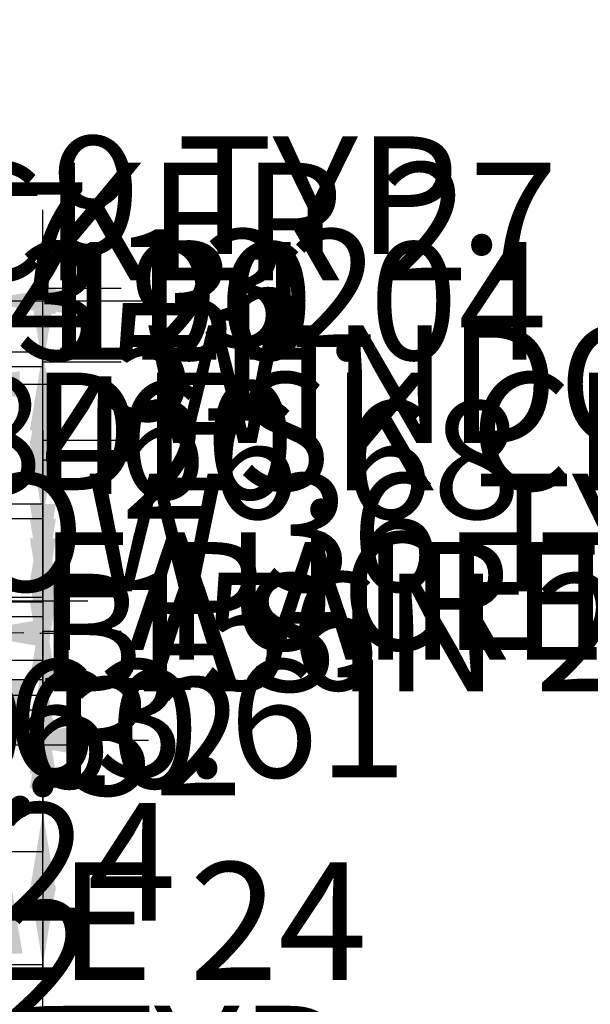
# Model space of a CAD drawing. Units: inches. Extents: x -307 to 2141, y -58 to 895.
# Tile 27 of 28: x 933 to 1283, y 292 to 895. Entities that reach past the tile are written whole.
import ezdxf

# ---------------------------------------------------------------- set-up
doc = ezdxf.new("R2010")
doc.units = ezdxf.units.IN
doc.header["$MEASUREMENT"] = 0
doc.layers.add('A-ANNO-DIMS', color=2, linetype='Continuous', lineweight=18)
doc.styles.get("Standard").update_dxf_attribs({"font": 'arial.ttf'})
doc.dimstyles.get("Standard").update_dxf_attribs({"dimtxt": 72, "dimasz": 48, "dimexe": 0.18, "dimexo": 0.0625, "dimgap": 0.09, "dimtad": 0, "dimtih": 1, "dimtoh": 1, "dimdec": 0, "dimrnd": 48, "dimzin": 0, "dimdsep": 46, "dimlunit": 3, "dimtxsty": 'Standard', "dimcen": 0.09, "dimadec": 0, "dimazin": 0, "dimtfac": 1, "dimtdec": 0, "dimtofl": 0, "dimtmove": 0, "dimatfit": 3, "dimfxl": 1, "dimtolj": 1, "dimtzin": 0, "dimarcsym": 0})

# ---------------------------------------------------------------- blocks, each defined once
blk = doc.blocks.new('*D29')
at = {"layer": 'A-ANNO-DIMS', "color": 0, "lineweight": -2, "transparency": 16777216}
for p, q in [((747.42, 450.87), (699.42, 450.87)), ((795.42, 433.61), (795.42, 451.05)), ((882.03, 433.61), (882.03, 451.05)), ((930.03, 450.87), (978.03, 450.87))]:
    blk.add_line(p, q, dxfattribs=at)
at = {"layer": 'A-ANNO-DIMS', "color": 0, "transparency": 16777216}
for points in [[(747.42, 458.87), (747.42, 442.87), (795.42, 450.87)], [(930.03, 458.87), (930.03, 442.87), (882.03, 450.87)]]:
    blk.add_solid(points, dxfattribs=at)
at = {"layer": 'Defpoints', "color": 0, "transparency": 16777216}
for p in [(795.42, 450.87), (795.42, 433.55), (882.03, 433.55)]:
    blk.add_point(p, dxfattribs=at)
at = {"layer": 'A-ANNO-DIMS', "color": 0, "transparency": 16777216, "insert": (647.71, 450.87), "char_height": 72, "attachment_point": 5}
blk.add_mtext('\\A1;87', dxfattribs=at)
blk = doc.blocks.new('*D30')
at = {"layer": 'A-ANNO-DIMS', "color": 0, "lineweight": -2, "transparency": 16777216}
for p, q in [((570.74, 532.83), (570.74, 580.83)), ((570.74, 580.83), (618.74, 580.83)), ((565.4, 484.83), (570.92, 484.83)), ((565.4, 448.83), (570.92, 448.83)), ((570.74, 400.83), (570.74, 352.83))]:
    blk.add_line(p, q, dxfattribs=at)
at = {"layer": 'A-ANNO-DIMS', "color": 0, "transparency": 16777216}
for points in [[(562.74, 532.83), (578.74, 532.83), (570.74, 484.83)], [(562.74, 400.83), (578.74, 400.83), (570.74, 448.83)]]:
    blk.add_solid(points, dxfattribs=at)
at = {"layer": 'Defpoints', "color": 0, "transparency": 16777216}
for p in [(565.34, 484.83), (570.74, 484.83), (565.34, 448.83)]:
    blk.add_point(p, dxfattribs=at)
at = {"layer": 'A-ANNO-DIMS', "color": 0, "transparency": 16777216, "insert": (1030.17, 580.83), "char_height": 72, "attachment_point": 5}
blk.add_mtext('\\A1;WINDOW 36 TYP.', dxfattribs=at)
blk = doc.blocks.new('*D31')
at = {"layer": 'A-ANNO-DIMS', "color": 0, "lineweight": -2, "transparency": 16777216}
for p, q in [((556.34, 448.77), (556.34, 443.25)), ((565.34, 448.77), (565.34, 443.25)), ((508.34, 443.43), (460.34, 443.43)), ((613.34, 443.43), (661.34, 443.43))]:
    blk.add_line(p, q, dxfattribs=at)
at = {"layer": 'A-ANNO-DIMS', "color": 0, "transparency": 16777216}
for points in [[(508.34, 451.43), (508.34, 435.43), (556.34, 443.43)], [(613.34, 451.43), (613.34, 435.43), (565.34, 443.43)]]:
    blk.add_solid(points, dxfattribs=at)
at = {"layer": 'Defpoints', "color": 0, "transparency": 16777216}
for p in [(556.34, 448.83), (565.34, 448.83), (565.34, 443.43)]:
    blk.add_point(p, dxfattribs=at)
at = {"layer": 'A-ANNO-DIMS', "color": 0, "transparency": 16777216, "insert": (808.69, 443.43), "char_height": 72, "attachment_point": 5}
blk.add_mtext('\\A1;9 TYP.', dxfattribs=at)
blk = doc.blocks.new('*D32')
at = {"layer": 'A-ANNO-DIMS', "color": 0, "lineweight": -2, "transparency": 16777216}
for p, q in [((813.29, 682.28), (813.29, 671.36)), ((885.29, 682.28), (885.29, 671.36)), ((765.29, 671.54), (717.29, 671.54)), ((933.29, 671.54), (981.29, 671.54))]:
    blk.add_line(p, q, dxfattribs=at)
at = {"layer": 'A-ANNO-DIMS', "color": 0, "transparency": 16777216}
for points in [[(765.29, 679.54), (765.29, 663.54), (813.29, 671.54)], [(933.29, 679.54), (933.29, 663.54), (885.29, 671.54)]]:
    blk.add_solid(points, dxfattribs=at)
at = {"layer": 'Defpoints', "color": 0, "transparency": 16777216}
for p in [(813.29, 682.34), (885.29, 682.34), (885.29, 671.54)]:
    blk.add_point(p, dxfattribs=at)
at = {"layer": 'A-ANNO-DIMS', "color": 0, "transparency": 16777216, "insert": (1392.73, 671.54), "char_height": 72, "attachment_point": 5}
blk.add_mtext('\\A1;WINDOW 72 TYP.', dxfattribs=at)
blk = doc.blocks.new('*D33')
at = {"layer": 'A-ANNO-DIMS', "color": 0, "lineweight": -2, "transparency": 16777216}
for p, q in [((896.09, 739.34), (896.09, 787.34)), ((896.09, 787.34), (944.09, 787.34)), ((885.36, 691.34), (896.27, 691.34)), ((885.36, 682.34), (896.27, 682.34)), ((896.09, 634.34), (896.09, 586.34))]:
    blk.add_line(p, q, dxfattribs=at)
at = {"layer": 'A-ANNO-DIMS', "color": 0, "transparency": 16777216}
for points in [[(888.09, 739.34), (904.09, 739.34), (896.09, 691.34)], [(888.09, 634.34), (904.09, 634.34), (896.09, 682.34)]]:
    blk.add_solid(points, dxfattribs=at)
at = {"layer": 'Defpoints', "color": 0, "transparency": 16777216}
for p in [(885.29, 691.34), (896.09, 691.34), (885.29, 682.34)]:
    blk.add_point(p, dxfattribs=at)
at = {"layer": 'A-ANNO-DIMS', "color": 0, "transparency": 16777216, "insert": (1091.45, 787.34), "char_height": 72, "attachment_point": 5}
blk.add_mtext('\\A1;9 TYP.', dxfattribs=at)
blk = doc.blocks.new('*D34')
at = {"layer": 'A-ANNO-DIMS', "color": 0, "lineweight": -2, "transparency": 16777216}
for p, q in [((927.14, 490.97), (927.14, 538.97)), ((927.14, 538.97), (975.14, 538.97)), ((916.4, 442.97), (927.32, 442.97)), ((916.4, 370.95), (927.32, 370.95)), ((927.14, 322.95), (927.14, 274.95))]:
    blk.add_line(p, q, dxfattribs=at)
at = {"layer": 'A-ANNO-DIMS', "color": 0, "transparency": 16777216}
for points in [[(919.14, 490.97), (935.14, 490.97), (927.14, 442.97)], [(919.14, 322.95), (935.14, 322.95), (927.14, 370.95)]]:
    blk.add_solid(points, dxfattribs=at)
at = {"layer": 'Defpoints', "color": 0, "transparency": 16777216}
for p in [(916.34, 442.97), (927.14, 442.97), (916.34, 370.95)]:
    blk.add_point(p, dxfattribs=at)
at = {"layer": 'A-ANNO-DIMS', "color": 0, "transparency": 16777216, "insert": (1584.53, 538.97), "char_height": 72, "attachment_point": 5}
blk.add_mtext('\\A1;PAIRED WINDOW 72 TYP.', dxfattribs=at)
blk = doc.blocks.new('*D35')
at = {"layer": 'A-ANNO-DIMS', "color": 0, "lineweight": -2, "transparency": 16777216}
for p, q in [((859.34, 453.77), (811.34, 453.77)), ((907.34, 443.03), (907.34, 453.95)), ((916.34, 443.03), (916.34, 453.95)), ((964.34, 453.77), (1012.34, 453.77))]:
    blk.add_line(p, q, dxfattribs=at)
at = {"layer": 'A-ANNO-DIMS', "color": 0, "transparency": 16777216}
for points in [[(859.34, 461.77), (859.34, 445.77), (907.34, 453.77)], [(964.34, 461.77), (964.34, 445.77), (916.34, 453.77)]]:
    blk.add_solid(points, dxfattribs=at)
at = {"layer": 'Defpoints', "color": 0, "transparency": 16777216}
for p in [(907.34, 453.77), (907.34, 442.97), (916.34, 442.97)]:
    blk.add_point(p, dxfattribs=at)
at = {"layer": 'A-ANNO-DIMS', "color": 0, "transparency": 16777216, "insert": (663.98, 453.77), "char_height": 72, "attachment_point": 5}
blk.add_mtext('\\A1;9 TYP.', dxfattribs=at)
blk = doc.blocks.new('*D37')
at = {"layer": 'A-ANNO-DIMS', "color": 0, "lineweight": -2, "transparency": 16777216}
for p, q in [((828.62, 519.41), (780.62, 519.46)), ((876.61, 514.46), (876.62, 519.54)), ((897.61, 514.44), (897.62, 519.51)), ((945.62, 519.28), (993.62, 519.22))]:
    blk.add_line(p, q, dxfattribs=at)
at = {"layer": 'A-ANNO-DIMS', "color": 0, "transparency": 16777216}
for points in [[(828.63, 527.41), (828.61, 511.41), (876.62, 519.36)], [(945.63, 527.28), (945.61, 511.28), (897.62, 519.33)]]:
    blk.add_solid(points, dxfattribs=at)
at = {"layer": 'Defpoints', "color": 0, "transparency": 16777216}
for p in [(876.62, 519.36), (876.61, 514.4), (897.61, 514.38)]:
    blk.add_point(p, dxfattribs=at)
at = {"layer": 'A-ANNO-DIMS', "color": 0, "transparency": 16777216, "insert": (604.68, 519.46), "char_height": 72, "attachment_point": 5}
blk.add_mtext('\\A1;21 TYP.', dxfattribs=at)
blk = doc.blocks.new('*D41')
at = {"layer": 'A-ANNO-DIMS', "color": 0, "lineweight": -2, "transparency": 16777216}
for p, q in [((768.38, 207.13), (768.38, 255.13)), ((768.38, 255.13), (816.38, 255.13)), ((762.83, 159.13), (768.56, 159.13)), ((762.83, 128.96), (768.56, 128.96)), ((768.38, 80.96), (768.38, 32.96))]:
    blk.add_line(p, q, dxfattribs=at)
at = {"layer": 'A-ANNO-DIMS', "color": 0, "transparency": 16777216}
for points in [[(760.38, 207.13), (776.38, 207.13), (768.38, 159.13)], [(760.38, 80.96), (776.38, 80.96), (768.38, 128.96)]]:
    blk.add_solid(points, dxfattribs=at)
at = {"layer": 'Defpoints', "color": 0, "transparency": 16777216}
for p in [(762.77, 159.13), (768.38, 159.13), (762.77, 128.96)]:
    blk.add_point(p, dxfattribs=at)
at = {"layer": 'A-ANNO-DIMS', "color": 0, "transparency": 16777216, "insert": (991.68, 255.13), "char_height": 72, "attachment_point": 5}
blk.add_mtext('\\A1;30 TYP.', dxfattribs=at)
blk = doc.blocks.new('*D42')
at = {"layer": 'A-ANNO-DIMS', "color": 0, "lineweight": -2, "transparency": 16777216}
for p, q in [((822.3, 541.2), (822.27, 542.82)), ((832.3, 541.41), (832.27, 543.03)), ((880.26, 543.86), (928.25, 544.87)), ((774.28, 541.63), (726.29, 540.62))]:
    blk.add_line(p, q, dxfattribs=at)
at = {"layer": 'A-ANNO-DIMS', "color": 0, "transparency": 16777216}
for points in [[(774.11, 549.63), (774.45, 533.63), (822.27, 542.64)], [(880.09, 551.86), (880.43, 535.86), (832.27, 542.85)]]:
    blk.add_solid(points, dxfattribs=at)
at = {"layer": 'Defpoints', "color": 0, "transparency": 16777216}
for p in [(832.27, 542.85), (822.3, 541.14), (832.3, 541.35)]:
    blk.add_point(p, dxfattribs=at)
at = {"layer": 'A-ANNO-DIMS', "color": 0, "transparency": 16777216, "insert": (1192.89, 544.87), "char_height": 72, "attachment_point": 5}
blk.add_mtext('\\A1;FAUCET 10', dxfattribs=at)
blk = doc.blocks.new('*D44')
at = {"layer": 'A-ANNO-DIMS', "color": 0, "lineweight": -2, "transparency": 16777216}
for p, q in [((815.33, 520.71), (815.41, 516.91)), ((839.87, 521.22), (839.95, 517.42)), ((887.94, 518.61), (935.93, 519.62)), ((767.41, 516.08), (719.42, 515.07))]:
    blk.add_line(p, q, dxfattribs=at)
at = {"layer": 'A-ANNO-DIMS', "color": 0, "transparency": 16777216}
for points in [[(887.77, 526.61), (888.11, 510.61), (839.95, 517.6)], [(767.25, 524.08), (767.58, 508.08), (815.4, 517.09)]]:
    blk.add_solid(points, dxfattribs=at)
at = {"layer": 'Defpoints', "color": 0, "transparency": 16777216}
for p in [(815.33, 520.77), (839.87, 521.29), (839.95, 517.6)]:
    blk.add_point(p, dxfattribs=at)
at = {"layer": 'A-ANNO-DIMS', "color": 0, "transparency": 16777216, "insert": (1151.16, 519.62), "char_height": 72, "attachment_point": 5}
blk.add_mtext('\\A1;BASIN 25', dxfattribs=at)
blk = doc.blocks.new('*D46')
at = {"layer": 'A-ANNO-DIMS', "color": 0, "lineweight": -2, "transparency": 16777216}
for p, q in [((801.41, 645.78), (801.41, 642.52)), ((822.41, 645.78), (822.41, 642.52)), ((753.41, 642.7), (705.41, 642.7)), ((870.41, 642.7), (918.41, 642.7))]:
    blk.add_line(p, q, dxfattribs=at)
at = {"layer": 'A-ANNO-DIMS', "color": 0, "transparency": 16777216}
for points in [[(753.41, 650.7), (753.41, 634.7), (801.41, 642.7)], [(870.41, 650.7), (870.41, 634.7), (822.41, 642.7)]]:
    blk.add_solid(points, dxfattribs=at)
at = {"layer": 'Defpoints', "color": 0, "transparency": 16777216}
for p in [(801.41, 645.85), (822.41, 645.85), (822.41, 642.7)]:
    blk.add_point(p, dxfattribs=at)
at = {"layer": 'A-ANNO-DIMS', "color": 0, "transparency": 16777216, "insert": (1282.7, 642.7), "char_height": 72, "attachment_point": 5}
blk.add_mtext('\\A1;DESK CHAIR 21', dxfattribs=at)
blk = doc.blocks.new('*D47')
at = {"layer": 'A-ANNO-DIMS', "color": 0, "lineweight": -2, "transparency": 16777216}
for p, q in [((825.56, 711.18), (825.56, 759.18)), ((825.56, 759.18), (873.56, 759.18)), ((822.48, 663.18), (825.74, 663.18)), ((822.48, 645.85), (825.74, 645.85)), ((825.56, 597.85), (825.56, 549.85))]:
    blk.add_line(p, q, dxfattribs=at)
at = {"layer": 'A-ANNO-DIMS', "color": 0, "transparency": 16777216}
for points in [[(817.56, 711.18), (833.56, 711.18), (825.56, 663.18)], [(817.56, 597.85), (833.56, 597.85), (825.56, 645.85)]]:
    blk.add_solid(points, dxfattribs=at)
at = {"layer": 'Defpoints', "color": 0, "transparency": 16777216}
for p in [(822.41, 663.18), (825.56, 663.18), (822.41, 645.85)]:
    blk.add_point(p, dxfattribs=at)
at = {"layer": 'A-ANNO-DIMS', "color": 0, "transparency": 16777216, "insert": (921.83, 759.18), "char_height": 72, "attachment_point": 5}
blk.add_mtext('\\A1;17', dxfattribs=at)
blk = doc.blocks.new('*D52')
at = {"layer": 'A-ANNO-DIMS', "color": 0, "lineweight": -2, "transparency": 16777216}
for p, q in [((660.21, 554.25), (660.21, 602.25)), ((673.8, 506.25), (660.03, 506.25)), ((673.8, 415.25), (660.03, 415.25)), ((660.21, 367.25), (660.21, 319.25))]:
    blk.add_line(p, q, dxfattribs=at)
at = {"layer": 'A-ANNO-DIMS', "color": 0, "transparency": 16777216}
for points in [[(652.21, 554.25), (668.21, 554.25), (660.21, 506.25)], [(652.21, 367.25), (668.21, 367.25), (660.21, 415.25)]]:
    blk.add_solid(points, dxfattribs=at)
at = {"layer": 'Defpoints', "color": 0, "transparency": 16777216}
for p in [(673.86, 506.25), (660.21, 415.25), (673.86, 415.25)]:
    blk.add_point(p, dxfattribs=at)
at = {"layer": 'A-ANNO-DIMS', "color": 0, "transparency": 16777216, "insert": (660.21, 460.75), "char_height": 72, "attachment_point": 5}
blk.add_mtext('\\A1;DINING SET 91', dxfattribs=at)
blk = doc.blocks.new('*D54')
at = {"layer": 'A-ANNO-DIMS', "color": 0, "lineweight": -2, "transparency": 16777216}
for p, q in [((605.34, 412.35), (605.34, 460.35)), ((605.34, 460.35), (653.34, 460.35)), ((596.4, 364.35), (605.52, 364.35)), ((596.4, 304.35), (605.52, 304.35)), ((605.34, 256.35), (605.34, 208.35))]:
    blk.add_line(p, q, dxfattribs=at)
at = {"layer": 'A-ANNO-DIMS', "color": 0, "transparency": 16777216}
for points in [[(597.34, 412.35), (613.34, 412.35), (605.34, 364.35)], [(597.34, 256.35), (613.34, 256.35), (605.34, 304.35)]]:
    blk.add_solid(points, dxfattribs=at)
at = {"layer": 'Defpoints', "color": 0, "transparency": 16777216}
for p in [(596.34, 364.35), (605.34, 364.35), (596.34, 304.35)]:
    blk.add_point(p, dxfattribs=at)
at = {"layer": 'A-ANNO-DIMS', "color": 0, "transparency": 16777216, "insert": (854, 460.35), "char_height": 72, "attachment_point": 5}
blk.add_mtext('\\A1;DESK 60', dxfattribs=at)
blk = doc.blocks.new('*D56')
at = {"layer": 'A-ANNO-DIMS', "color": 0, "lineweight": -2, "transparency": 16777216}
for p, q in [((679.73, 723.21), (679.73, 771.21)), ((679.73, 771.21), (727.73, 771.21)), ((675.74, 675.21), (679.91, 675.21)), ((675.74, 648.21), (679.91, 648.21)), ((679.73, 600.21), (679.73, 552.21))]:
    blk.add_line(p, q, dxfattribs=at)
at = {"layer": 'A-ANNO-DIMS', "color": 0, "transparency": 16777216}
for points in [[(671.73, 723.21), (687.73, 723.21), (679.73, 675.21)], [(671.73, 600.21), (687.73, 600.21), (679.73, 648.21)]]:
    blk.add_solid(points, dxfattribs=at)
at = {"layer": 'Defpoints', "color": 0, "transparency": 16777216}
for p in [(675.68, 675.21), (679.73, 675.21), (675.68, 648.21)]:
    blk.add_point(p, dxfattribs=at)
at = {"layer": 'A-ANNO-DIMS', "color": 0, "transparency": 16777216, "insert": (1006.66, 771.21), "char_height": 72, "attachment_point": 5}
blk.add_mtext('\\A1;ROCKER 27', dxfattribs=at)
blk = doc.blocks.new('*D60')
at = {"layer": 'A-ANNO-DIMS', "color": 0, "lineweight": -2, "transparency": 16777216}
for p, q in [((659.86, 294.95), (659.86, 342.95)), ((659.86, 342.95), (707.86, 342.95)), ((663.34, 246.95), (659.68, 246.95)), ((663.34, 223.32), (659.68, 223.32)), ((659.86, 175.32), (659.86, 127.32))]:
    blk.add_line(p, q, dxfattribs=at)
at = {"layer": 'A-ANNO-DIMS', "color": 0, "transparency": 16777216}
for points in [[(651.86, 294.95), (667.86, 294.95), (659.86, 246.95)], [(651.86, 175.32), (667.86, 175.32), (659.86, 223.32)]]:
    blk.add_solid(points, dxfattribs=at)
at = {"layer": 'Defpoints', "color": 0, "transparency": 16777216}
for p in [(659.86, 246.95), (663.4, 246.95), (663.4, 223.32)]:
    blk.add_point(p, dxfattribs=at)
at = {"layer": 'A-ANNO-DIMS', "color": 0, "transparency": 16777216, "insert": (933.57, 342.95), "char_height": 72, "attachment_point": 5}
blk.add_mtext('\\A1;TABLE 24', dxfattribs=at)
blk = doc.blocks.new('*D63')
at = {"layer": 'A-ANNO-DIMS', "color": 0, "lineweight": -2, "transparency": 16777216}
for p, q in [((916.4, 691.34), (947.72, 691.34)), ((947.54, 643.34), (947.54, 416.19)), ((947.54, 115.34), (947.54, 342.49)), ((704.68, 67.34), (947.72, 67.34))]:
    blk.add_line(p, q, dxfattribs=at)
at = {"layer": 'A-ANNO-DIMS', "color": 0, "transparency": 16777216}
for points in [[(939.54, 643.34), (955.54, 643.34), (947.54, 691.34)], [(939.54, 115.34), (955.54, 115.34), (947.54, 67.34)]]:
    blk.add_solid(points, dxfattribs=at)
at = {"layer": 'Defpoints', "color": 0, "transparency": 16777216}
for p in [(916.34, 691.34), (704.62, 67.34), (947.54, 67.34)]:
    blk.add_point(p, dxfattribs=at)
at = {"layer": 'A-ANNO-DIMS', "color": 0, "transparency": 16777216, "insert": (947.54, 379.34), "char_height": 72, "attachment_point": 5}
blk.add_mtext('\\A1;624', dxfattribs=at)
blk = doc.blocks.new('*D76')
at = {"layer": 'A-ANNO-DIMS', "color": 0, "lineweight": -2, "transparency": 16777216}
for p, q in [((646.34, 722.54), (598.34, 722.54)), ((694.34, 682.4), (694.34, 722.72)), ((778.34, 682.4), (778.34, 722.72)), ((826.34, 722.54), (874.34, 722.54))]:
    blk.add_line(p, q, dxfattribs=at)
at = {"layer": 'A-ANNO-DIMS', "color": 0, "transparency": 16777216}
for points in [[(646.34, 730.54), (646.34, 714.54), (694.34, 722.54)], [(826.34, 730.54), (826.34, 714.54), (778.34, 722.54)]]:
    blk.add_solid(points, dxfattribs=at)
at = {"layer": 'Defpoints', "color": 0, "transparency": 16777216}
for p in [(778.34, 722.54), (694.34, 682.34), (778.34, 682.34)]:
    blk.add_point(p, dxfattribs=at)
at = {"layer": 'A-ANNO-DIMS', "color": 0, "transparency": 16777216, "insert": (925.9, 722.54), "char_height": 72, "attachment_point": 5}
blk.add_mtext('\\A1;84', dxfattribs=at)
blk = doc.blocks.new('*D77')
at = {"layer": 'A-ANNO-DIMS', "color": 0, "lineweight": -2, "transparency": 16777216}
for p, q in [((787.34, 682.4), (787.34, 722.72)), ((835.34, 722.54), (859.34, 722.54)), ((907.34, 682.4), (907.34, 722.72)), ((907.34, 722.54), (955.34, 722.54))]:
    blk.add_line(p, q, dxfattribs=at)
at = {"layer": 'A-ANNO-DIMS', "color": 0, "transparency": 16777216}
for points in [[(835.34, 730.54), (835.34, 714.54), (787.34, 722.54)], [(859.34, 730.54), (859.34, 714.54), (907.34, 722.54)]]:
    blk.add_solid(points, dxfattribs=at)
at = {"layer": 'Defpoints', "color": 0, "transparency": 16777216}
for p in [(907.34, 722.54), (787.34, 682.34), (907.34, 682.34)]:
    blk.add_point(p, dxfattribs=at)
at = {"layer": 'A-ANNO-DIMS', "color": 0, "transparency": 16777216, "insert": (1031.45, 722.54), "char_height": 72, "attachment_point": 5}
blk.add_mtext('\\A1;120', dxfattribs=at)
blk = doc.blocks.new('*D78')
at = {"layer": 'A-ANNO-DIMS', "color": 0, "lineweight": -2, "transparency": 16777216}
for p, q in [((947.53984, 730.340828), (947.53984, 778.340828)), ((778.39834, 682.340828), (947.71984, 682.340828)), ((730.39834, 598.340828), (947.71984, 598.340828)), ((947.53984, 550.340828), (947.53984, 502.340828))]:
    blk.add_line(p, q, dxfattribs=at)
at = {"layer": 'A-ANNO-DIMS', "color": 0, "transparency": 16777216}
for points in [[(939.53984, 730.340828), (955.53984, 730.340828), (947.53984, 682.340828)], [(939.53984, 550.340828), (955.53984, 550.340828), (947.53984, 598.340828)]]:
    blk.add_solid(points, dxfattribs=at)
at = {"layer": 'Defpoints', "color": 0, "transparency": 16777216}
for p in [(778.33584, 682.340828), (947.53984, 682.340828), (730.33584, 598.340828)]:
    blk.add_point(p, dxfattribs=at)
at = {"layer": 'A-ANNO-DIMS', "color": 0, "transparency": 16777216, "insert": (947.53984, 640.340828), "char_height": 72, "attachment_point": 5}
blk.add_mtext('\\A1;84', dxfattribs=at)
blk = doc.blocks.new('*D79')
at = {"layer": 'A-ANNO-DIMS', "color": 0, "lineweight": -2, "transparency": 16777216}
for p, q in [((947.54, 682.34), (947.54, 730.34)), ((947.54, 730.34), (995.54, 730.34)), ((907.4, 682.34), (947.72, 682.34)), ((947.54, 598.34), (947.54, 634.34)), ((907.4, 550.34), (947.72, 550.34))]:
    blk.add_line(p, q, dxfattribs=at)
at = {"layer": 'A-ANNO-DIMS', "color": 0, "transparency": 16777216}
for points in [[(939.54, 634.34), (955.54, 634.34), (947.54, 682.34)], [(939.54, 598.34), (955.54, 598.34), (947.54, 550.34)]]:
    blk.add_solid(points, dxfattribs=at)
at = {"layer": 'Defpoints', "color": 0, "transparency": 16777216}
for p in [(907.34, 682.34), (947.54, 682.34), (907.34, 550.34)]:
    blk.add_point(p, dxfattribs=at)
at = {"layer": 'A-ANNO-DIMS', "color": 0, "transparency": 16777216, "insert": (1071.41, 730.34), "char_height": 72, "attachment_point": 5}
blk.add_mtext('\\A1;132', dxfattribs=at)
blk = doc.blocks.new('*D80')
at = {"layer": 'A-ANNO-DIMS', "color": 0, "lineweight": -2, "transparency": 16777216}
for p, q in [((763.34, 722.54), (715.34, 722.54)), ((811.34, 517.4), (811.34, 722.72)), ((907.34, 541.4), (907.34, 722.72)), ((955.34, 722.54), (1003.34, 722.54))]:
    blk.add_line(p, q, dxfattribs=at)
at = {"layer": 'A-ANNO-DIMS', "color": 0, "transparency": 16777216}
for points in [[(763.34, 730.54), (763.34, 714.54), (811.34, 722.54)], [(955.34, 730.54), (955.34, 714.54), (907.34, 722.54)]]:
    blk.add_solid(points, dxfattribs=at)
at = {"layer": 'Defpoints', "color": 0, "transparency": 16777216}
for p in [(907.34, 722.54), (907.34, 541.34), (811.34, 517.34)]:
    blk.add_point(p, dxfattribs=at)
at = {"layer": 'A-ANNO-DIMS', "color": 0, "transparency": 16777216, "insert": (1054.97, 722.54), "char_height": 72, "attachment_point": 5}
blk.add_mtext('\\A1;96', dxfattribs=at)
blk = doc.blocks.new('*D81')
at = {"layer": 'A-ANNO-DIMS', "color": 0, "lineweight": -2, "transparency": 16777216}
for p, q in [((947.54, 589.34), (947.54, 637.34)), ((947.54, 637.34), (995.54, 637.34)), ((907.4, 541.34), (947.72, 541.34)), ((907.4, 481.34), (947.72, 481.34)), ((947.54, 433.34), (947.54, 385.34))]:
    blk.add_line(p, q, dxfattribs=at)
at = {"layer": 'A-ANNO-DIMS', "color": 0, "transparency": 16777216}
for points in [[(939.54, 589.34), (955.54, 589.34), (947.54, 541.34)], [(939.54, 433.34), (955.54, 433.34), (947.54, 481.34)]]:
    blk.add_solid(points, dxfattribs=at)
at = {"layer": 'Defpoints', "color": 0, "transparency": 16777216}
for p in [(907.34, 541.34), (947.54, 541.34), (907.34, 481.34)]:
    blk.add_point(p, dxfattribs=at)
at = {"layer": 'A-ANNO-DIMS', "color": 0, "transparency": 16777216, "insert": (1047.27, 637.34), "char_height": 72, "attachment_point": 5}
blk.add_mtext('\\A1;60', dxfattribs=at)
blk = doc.blocks.new('*D83')
at = {"layer": 'A-ANNO-DIMS', "color": 0, "lineweight": -2, "transparency": 16777216}
for p, q in [((947.54, 538.9), (947.54, 586.9)), ((916.4, 490.9), (947.72, 490.9)), ((907.4, 481.34), (947.72, 481.34)), ((947.54, 433.34), (947.54, 385.34)), ((947.54, 385.34), (899.54, 385.34))]:
    blk.add_line(p, q, dxfattribs=at)
at = {"layer": 'A-ANNO-DIMS', "color": 0, "transparency": 16777216}
for points in [[(939.54, 538.9), (955.54, 538.9), (947.54, 490.9)], [(939.54, 433.34), (955.54, 433.34), (947.54, 481.34)]]:
    blk.add_solid(points, dxfattribs=at)
at = {"layer": 'Defpoints', "color": 0, "transparency": 16777216}
for p in [(916.34, 490.9), (907.34, 481.34), (947.54, 481.34)]:
    blk.add_point(p, dxfattribs=at)
at = {"layer": 'A-ANNO-DIMS', "color": 0, "transparency": 16777216, "insert": (777.97, 385.34), "char_height": 72, "attachment_point": 5}
blk.add_mtext('\\A1;9.563', dxfattribs=at)
blk = doc.blocks.new('*D84')
at = {"layer": 'A-ANNO-DIMS', "color": 0, "lineweight": -2, "transparency": 16777216}
for p, q in [((763.34, 472.28), (763.34, 35.96)), ((907.34, 472.28), (907.34, 35.96)), ((811.34, 36.14), (859.34, 36.14)), ((907.34, 36.14), (955.34, 36.14))]:
    blk.add_line(p, q, dxfattribs=at)
at = {"layer": 'A-ANNO-DIMS', "color": 0, "transparency": 16777216}
for points in [[(811.34, 44.14), (811.34, 28.14), (763.34, 36.14)], [(859.34, 44.14), (859.34, 28.14), (907.34, 36.14)]]:
    blk.add_solid(points, dxfattribs=at)
at = {"layer": 'Defpoints', "color": 0, "transparency": 16777216}
for p in [(763.34, 472.34), (907.34, 472.34), (907.34, 36.14)]:
    blk.add_point(p, dxfattribs=at)
at = {"layer": 'A-ANNO-DIMS', "color": 0, "transparency": 16777216, "insert": (1031.43, 36.14), "char_height": 72, "attachment_point": 5}
blk.add_mtext('\\A1;144', dxfattribs=at)
blk = doc.blocks.new('*D85')
at = {"layer": 'A-ANNO-DIMS', "color": 0, "lineweight": -2, "transparency": 16777216}
for p, q in [((947.54, 472.34), (947.54, 520.34)), ((947.54, 520.34), (995.54, 520.34)), ((907.4, 472.34), (947.72, 472.34)), ((947.54, 364.34), (947.54, 424.34)), ((916.4, 316.34), (947.72, 316.34))]:
    blk.add_line(p, q, dxfattribs=at)
at = {"layer": 'A-ANNO-DIMS', "color": 0, "transparency": 16777216}
for points in [[(939.54, 424.34), (955.54, 424.34), (947.54, 472.34)], [(939.54, 364.34), (955.54, 364.34), (947.54, 316.34)]]:
    blk.add_solid(points, dxfattribs=at)
at = {"layer": 'Defpoints', "color": 0, "transparency": 16777216}
for p in [(907.34, 472.34), (947.54, 472.34), (916.34, 316.34)]:
    blk.add_point(p, dxfattribs=at)
at = {"layer": 'A-ANNO-DIMS', "color": 0, "transparency": 16777216, "insert": (1071.76, 520.34), "char_height": 72, "attachment_point": 5}
blk.add_mtext('\\A1;156', dxfattribs=at)
blk = doc.blocks.new('*D95')
at = {"layer": 'A-ANNO-DIMS', "color": 0, "lineweight": -2, "transparency": 16777216}
for p, q in [((947.54, 577.34), (947.54, 625.34)), ((947.54, 625.34), (995.54, 625.34)), ((629.9, 529.34), (947.72, 529.34)), ((629.9, 502.66), (947.72, 502.66)), ((947.54, 454.66), (947.54, 406.66))]:
    blk.add_line(p, q, dxfattribs=at)
at = {"layer": 'A-ANNO-DIMS', "color": 0, "transparency": 16777216}
for points in [[(939.54, 577.34), (955.54, 577.34), (947.54, 529.34)], [(939.54, 454.66), (955.54, 454.66), (947.54, 502.66)]]:
    blk.add_solid(points, dxfattribs=at)
at = {"layer": 'Defpoints', "color": 0, "transparency": 16777216}
for p in [(629.84, 529.34), (947.54, 529.34), (629.84, 502.66)]:
    blk.add_point(p, dxfattribs=at)
at = {"layer": 'A-ANNO-DIMS', "color": 0, "transparency": 16777216, "insert": (1117.8, 625.34), "char_height": 72, "attachment_point": 5}
blk.add_mtext('\\A1;26.68', dxfattribs=at)
blk = doc.blocks.new('*D97')
at = {"layer": 'A-ANNO-DIMS', "color": 0, "lineweight": -2, "transparency": 16777216}
for p, q in [((947.54, 637.34), (947.54, 685.34)), ((947.54, 685.34), (995.54, 685.34)), ((685.4, 589.34), (947.72, 589.34)), ((685.4, 538.34), (947.72, 538.34)), ((947.54, 490.34), (947.54, 442.34))]:
    blk.add_line(p, q, dxfattribs=at)
at = {"layer": 'A-ANNO-DIMS', "color": 0, "transparency": 16777216}
for points in [[(939.54, 637.34), (955.54, 637.34), (947.54, 589.34)], [(939.54, 490.34), (955.54, 490.34), (947.54, 538.34)]]:
    blk.add_solid(points, dxfattribs=at)
at = {"layer": 'Defpoints', "color": 0, "transparency": 16777216}
for p in [(685.34, 589.34), (947.54, 589.34), (685.34, 538.34)]:
    blk.add_point(p, dxfattribs=at)
at = {"layer": 'A-ANNO-DIMS', "color": 0, "transparency": 16777216, "insert": (1040.25, 685.34), "char_height": 72, "attachment_point": 5}
blk.add_mtext('\\A1;51', dxfattribs=at)
blk = doc.blocks.new('*D99')
at = {"layer": 'A-ANNO-DIMS', "color": 0, "lineweight": -2, "transparency": 16777216}
for p, q in [((763.34, 481.28), (763.34, 35.96)), ((802.34, 481.28), (802.34, 35.96)), ((715.34, 36.14), (667.34, 36.14)), ((850.34, 36.14), (898.34, 36.14))]:
    blk.add_line(p, q, dxfattribs=at)
at = {"layer": 'A-ANNO-DIMS', "color": 0, "transparency": 16777216}
for points in [[(715.34, 44.14), (715.34, 28.14), (763.34, 36.14)], [(850.34, 44.14), (850.34, 28.14), (802.34, 36.14)]]:
    blk.add_solid(points, dxfattribs=at)
at = {"layer": 'Defpoints', "color": 0, "transparency": 16777216}
for p in [(763.34, 481.34), (802.34, 481.34), (802.34, 36.14)]:
    blk.add_point(p, dxfattribs=at)
at = {"layer": 'A-ANNO-DIMS', "color": 0, "transparency": 16777216, "insert": (950.04, 36.14), "char_height": 72, "attachment_point": 5}
blk.add_mtext('\\A1;39', dxfattribs=at)
blk = doc.blocks.new('*D102')
at = {"layer": 'A-ANNO-DIMS', "color": 0, "lineweight": -2, "transparency": 16777216}
for p, q in [((837.29, 722.54), (789.29, 722.54)), ((885.29, 691.4), (885.29, 722.72)), ((916.34, 691.4), (916.34, 722.72)), ((964.34, 722.54), (1012.34, 722.54))]:
    blk.add_line(p, q, dxfattribs=at)
at = {"layer": 'A-ANNO-DIMS', "color": 0, "transparency": 16777216}
for points in [[(837.29, 730.54), (837.29, 714.54), (885.29, 722.54)], [(964.34, 730.54), (964.34, 714.54), (916.34, 722.54)]]:
    blk.add_solid(points, dxfattribs=at)
at = {"layer": 'Defpoints', "color": 0, "transparency": 16777216}
for p in [(916.34, 722.54), (885.29, 691.34), (916.34, 691.34)]:
    blk.add_point(p, dxfattribs=at)
at = {"layer": 'A-ANNO-DIMS', "color": 0, "transparency": 16777216, "insert": (1133.74, 722.54), "char_height": 72, "attachment_point": 5}
blk.add_mtext('\\A1;31.04', dxfattribs=at)
blk = doc.blocks.new('*D104')
at = {"layer": 'A-ANNO-DIMS', "color": 0, "lineweight": -2, "transparency": 16777216}
for p, q in [((885.13, 418.95), (885.13, 466.95)), ((885.13, 466.95), (933.13, 466.95)), ((916.27, 370.95), (884.95, 370.95)), ((916.27, 307.34), (884.95, 307.34)), ((885.13, 259.34), (885.13, 211.34))]:
    blk.add_line(p, q, dxfattribs=at)
at = {"layer": 'A-ANNO-DIMS', "color": 0, "transparency": 16777216}
for points in [[(877.13, 418.95), (893.13, 418.95), (885.13, 370.95)], [(877.13, 259.34), (893.13, 259.34), (885.13, 307.34)]]:
    blk.add_solid(points, dxfattribs=at)
at = {"layer": 'Defpoints', "color": 0, "transparency": 16777216}
for p in [(885.13, 370.95), (916.34, 370.95), (916.34, 307.34)]:
    blk.add_point(p, dxfattribs=at)
at = {"layer": 'A-ANNO-DIMS', "color": 0, "transparency": 16777216, "insert": (1047.95, 466.95), "char_height": 72, "attachment_point": 5}
blk.add_mtext('\\A1;63.61', dxfattribs=at)
blk = doc.blocks.new('*D105')
at = {"layer": 'A-ANNO-DIMS', "color": 0, "lineweight": -2, "transparency": 16777216}
for p, q in [((828.13, 271.34), (828.13, 319.34)), ((828.13, 319.34), (876.13, 319.34)), ((859.27, 223.34), (827.95, 223.34)), ((859.27, 211.34), (827.95, 211.34)), ((828.13, 163.34), (828.13, 115.34))]:
    blk.add_line(p, q, dxfattribs=at)
at = {"layer": 'A-ANNO-DIMS', "color": 0, "transparency": 16777216}
for points in [[(820.13, 271.34), (836.13, 271.34), (828.13, 223.34)], [(820.13, 163.34), (836.13, 163.34), (828.13, 211.34)]]:
    blk.add_solid(points, dxfattribs=at)
at = {"layer": 'Defpoints', "color": 0, "transparency": 16777216}
for p in [(828.13, 223.34), (859.34, 223.34), (859.34, 211.34)]:
    blk.add_point(p, dxfattribs=at)
at = {"layer": 'A-ANNO-DIMS', "color": 0, "transparency": 16777216, "insert": (924.03, 319.34), "char_height": 72, "attachment_point": 5}
blk.add_mtext('\\A1;12', dxfattribs=at)
blk = doc.blocks.new('*D107')
at = {"layer": 'A-ANNO-DIMS', "color": 0, "lineweight": -2, "transparency": 16777216}
for p, q in [((517.34, 722.54), (469.34, 722.54)), ((565.34, 409.4), (565.34, 722.72)), ((589.34, 409.4), (589.34, 722.72)), ((637.34, 722.54), (685.34, 722.54))]:
    blk.add_line(p, q, dxfattribs=at)
at = {"layer": 'A-ANNO-DIMS', "color": 0, "transparency": 16777216}
for points in [[(517.34, 730.54), (517.34, 714.54), (565.34, 722.54)], [(637.34, 730.54), (637.34, 714.54), (589.34, 722.54)]]:
    blk.add_solid(points, dxfattribs=at)
at = {"layer": 'Defpoints', "color": 0, "transparency": 16777216}
for p in [(589.34, 722.54), (565.34, 409.34), (589.34, 409.34)]:
    blk.add_point(p, dxfattribs=at)
at = {"layer": 'A-ANNO-DIMS', "color": 0, "transparency": 16777216, "insert": (835.49, 722.54), "char_height": 72, "attachment_point": 5}
blk.add_mtext('\\A1;24.003', dxfattribs=at)
blk = doc.blocks.new('*D108')
at = {"layer": 'A-ANNO-DIMS', "color": 0, "lineweight": -2, "transparency": 16777216}
for p, q in [((947.54, 550.66), (947.54, 598.66)), ((589.4, 502.66), (947.72, 502.66)), ((589.4, 409.34), (947.72, 409.34)), ((947.54, 361.34), (947.54, 313.34))]:
    blk.add_line(p, q, dxfattribs=at)
at = {"layer": 'A-ANNO-DIMS', "color": 0, "transparency": 16777216}
for points in [[(939.54, 550.66), (955.54, 550.66), (947.54, 502.66)], [(939.54, 361.34), (955.54, 361.34), (947.54, 409.34)]]:
    blk.add_solid(points, dxfattribs=at)
at = {"layer": 'Defpoints', "color": 0, "transparency": 16777216}
for p in [(589.34, 502.66), (947.54, 502.66), (589.34, 409.34)]:
    blk.add_point(p, dxfattribs=at)
at = {"layer": 'A-ANNO-DIMS', "color": 0, "transparency": 16777216, "insert": (947.54, 456), "char_height": 72, "attachment_point": 5}
blk.add_mtext('\\A1;93.32', dxfattribs=at)

msp = doc.modelspace()

# ---------------------------------------------------------------- dimensions: what is measured, and where the dimension line sits
at = {"layer": 'A-ANNO-DIMS'}
for base, p1, p2, angle, text, picture, middle in [((896.0934, 691.3408), (885.2934, 682.3408), (885.2934, 691.3408), 90, '<> TYP.', '*D33', (1091.4494, 787.3408)), ((679.7317, 675.211), (675.6817, 648.211), (675.6817, 675.211), 90, 'ROCKER <>', '*D56', (1006.6621, 771.211)), ((927.1381, 442.9669), (916.3358, 370.9517), (916.3358, 442.9669), 90, 'PAIRED WINDOW <> TYP.', '*D34', (1584.5269, 538.9669)), ((570.7358, 484.8333), (565.3358, 448.8333), (565.3358, 484.8333), 90, 'WINDOW <> TYP.', '*D30', (1030.1737, 580.8333)), ((832.2692, 542.8502), (822.3029, 541.1403), (832.3007, 541.3505), 1.2046277, 'FAUCET <>', '*D42', (1192.8864, 544.8684)), ((660.2083, 415.2485), (673.8583, 506.2485), (673.8583, 415.2485), 270, 'DINING SET <>', '*D52', (660.2083, 460.7485)), ((876.6162, 519.3557), (897.6106, 514.3753), (876.6106, 514.3988), 179.9358924, '<> TYP.', '*D37', (604.6763, 519.4631)), ((839.9481, 517.6035), (815.3253, 520.7692), (839.8707, 521.2853), 1.2046277, 'BASIN <>', '*D44', (1151.1574, 519.6217)), ((605.3358, 364.3488), (596.3358, 304.3488), (596.3358, 364.3488), 90, 'DESK <>', '*D54', (854.0043, 460.3488)), ((907.3358, 453.7692), (916.3358, 442.9669), (907.3358, 442.9669), 180, '<> TYP.', '*D35', (663.9798, 453.7692)), ((659.8571, 246.9465), (663.4018, 223.3153), (663.4018, 246.9465), 90, 'TABLE <>', '*D60', (933.5733, 342.9465)), ((768.3792, 159.1282), (762.7703, 128.9569), (762.7703, 159.1282), 90, '<> TYP.', '*D41', (991.6806, 255.1282))]:
    dim = msp.add_linear_dim(base=base, p1=p1, p2=p2, angle=angle, text=text, dimstyle='Standard', override={"dimdec": 0, "dimlfac": 1, "dimrnd": 0, "dimzin": 0, "dimdsep": 46, "dimlunit": 2}, dxfattribs=at)
    dim.commit()
    dim.dimension.update_dxf_attribs({"geometry": picture, "text_midpoint": middle})
for base, p1, p2, text, picture, middle in [((885.2934, 671.5408), (813.2934, 682.3408), (885.2934, 682.3408), 'WINDOW <> TYP.', '*D32', (1392.7312, 671.5408)), ((822.4132, 642.696), (801.4132, 645.846), (822.4132, 645.846), 'DESK CHAIR <>', '*D46', (1282.7024, 642.696)), ((565.3358, 443.4333), (556.3358, 448.8333), (565.3358, 448.8333), '<> TYP.', '*D31', (808.6919, 443.4333))]:
    dim = msp.add_linear_dim(base=base, p1=p1, p2=p2, text=text, dimstyle='Standard', override={"dimdec": 0, "dimlfac": 1, "dimrnd": 0, "dimzin": 0, "dimdsep": 46, "dimlunit": 2}, dxfattribs=at)
    dim.commit()
    dim.dimension.update_dxf_attribs({"geometry": picture, "text_midpoint": middle})
for base, p1, p2, angle, override, picture, middle in [((825.5632, 663.1793), (822.4132, 645.846), (822.4132, 663.1793), 90, {"dimdec": 0, "dimlfac": 1, "dimrnd": 0, "dimzin": 0, "dimdsep": 46, "dimlunit": 2}, '*D47', (921.8333, 759.1793)), ((947.5398, 682.3408), (730.3358, 598.3408), (778.3358, 682.3408), 90, {"dimdec": 0, "dimlfac": 1, "dimrnd": 0, "dimzin": 0, "dimdsep": 46, "dimlunit": 2}, '*D78', (947.5398, 640.3408)), ((947.5398, 682.3408), (907.3358, 550.3408), (907.3358, 682.3408), 90, {"dimdec": 0, "dimlfac": 1, "dimrnd": 0, "dimzin": 0, "dimdsep": 46, "dimlunit": 2}, '*D79', (1071.4116, 730.3408)), ((947.5398, 589.3408), (685.3358, 538.3408), (685.3358, 589.3408), 90, {"dimdec": 0, "dimlfac": 1, "dimrnd": 0, "dimzin": 0, "dimdsep": 46, "dimlunit": 2}, '*D97', (1040.2492, 685.3408)), ((947.5398, 67.3408), (916.3358, 691.3408), (704.6211, 67.3408), 90, {"dimdec": 0, "dimlfac": 1, "dimrnd": 0, "dimzin": 0, "dimdsep": 46, "dimlunit": 2}, '*D63', (947.5398, 379.3408)), ((947.5398, 541.3408), (907.3358, 481.3408), (907.3358, 541.3408), 90, {"dimdec": 0, "dimlfac": 1, "dimrnd": 0, "dimzin": 0, "dimdsep": 46, "dimlunit": 2}, '*D81', (1047.2724, 637.3408)), ((947.5398, 529.3408), (629.8358, 502.6632), (629.8358, 529.3408), 90, {"dimdec": 2, "dimlfac": 1, "dimrnd": 0, "dimzin": 0, "dimdsep": 46, "dimlunit": 2}, '*D95', (1117.799, 625.3408)), ((947.5398, 502.6632), (589.339, 409.3408), (589.339, 502.6632), 90, {"dimdec": 2, "dimlfac": 1, "dimrnd": 0, "dimzin": 0, "dimdsep": 46, "dimlunit": 2}, '*D108', (947.5398, 456.002)), ((947.5398, 481.3408), (916.3358, 490.9034), (907.3358, 481.3408), 90, {"dimdec": 3, "dimlfac": 1, "dimrnd": 0, "dimzin": 0, "dimdsep": 46, "dimlunit": 2}, '*D83', (777.9683, 385.3408)), ((947.5398, 472.3408), (916.3358, 316.3408), (907.3358, 472.3408), 90, {"dimdec": 0, "dimlfac": 1, "dimrnd": 0, "dimzin": 0, "dimdsep": 46, "dimlunit": 2}, '*D85', (1071.7554, 520.3408)), ((885.1318, 370.9517), (916.3358, 307.3408), (916.3358, 370.9517), 90, {"dimdec": 2, "dimlfac": 1, "dimrnd": 0, "dimzin": 0, "dimdsep": 46, "dimlunit": 2}, '*D104', (1047.9504, 466.9517)), ((795.4208, 450.8711), (882.0282, 433.5496), (795.4208, 433.5496), 180, {"dimdec": 0, "dimlfac": 1, "dimrnd": 0, "dimzin": 0, "dimdsep": 46, "dimlunit": 2}, '*D29', (647.7128, 450.8711)), ((828.1318, 223.3408), (859.3358, 211.3408), (859.3358, 223.3408), 90, {"dimdec": 0, "dimlfac": 1, "dimrnd": 0, "dimzin": 0, "dimdsep": 46, "dimlunit": 2}, '*D105', (924.0336, 319.3408))]:
    dim = msp.add_linear_dim(base=base, p1=p1, p2=p2, angle=angle, dimstyle='Standard', override=override, dxfattribs=at)
    dim.commit()
    dim.dimension.update_dxf_attribs({"geometry": picture, "text_midpoint": middle})
for base, p1, p2, override, picture, middle in [((589.339, 722.5448), (565.3358, 409.3408), (589.339, 409.3408), {"dimdec": 3, "dimlfac": 1, "dimrnd": 0, "dimzin": 0, "dimdsep": 46, "dimlunit": 2}, '*D107', (835.4945, 722.5448)), ((778.3358, 722.5448), (694.3358, 682.3408), (778.3358, 682.3408), {"dimdec": 0, "dimlfac": 1, "dimrnd": 0, "dimzin": 0, "dimdsep": 46, "dimlunit": 2}, '*D76', (925.8965, 722.5448)), ((907.3358, 722.5448), (811.3358, 517.3408), (907.3358, 541.3408), {"dimdec": 0, "dimlfac": 1, "dimrnd": 0, "dimzin": 0, "dimdsep": 46, "dimlunit": 2}, '*D80', (1054.9702, 722.5448)), ((907.3358, 722.5448), (787.3358, 682.3408), (907.3358, 682.3408), {"dimdec": 0, "dimlfac": 1, "dimrnd": 0, "dimzin": 0, "dimdsep": 46, "dimlunit": 2}, '*D77', (1031.4531, 722.5448)), ((916.3358, 722.5448), (885.2934, 691.3408), (916.3358, 691.3408), {"dimdec": 2, "dimlfac": 1, "dimrnd": 0, "dimzin": 0, "dimdsep": 46, "dimlunit": 2}, '*D102', (1133.7355, 722.5448)), ((802.3358, 36.1368), (763.3358, 481.3408), (802.3358, 481.3408), {"dimdec": 0, "dimlfac": 1, "dimrnd": 0, "dimzin": 0, "dimdsep": 46, "dimlunit": 2}, '*D99', (950.0438, 36.1368)), ((907.3358, 36.1368), (763.3358, 472.3408), (907.3358, 472.3408), {"dimdec": 0, "dimlfac": 1, "dimrnd": 0, "dimzin": 0, "dimdsep": 46, "dimlunit": 2}, '*D84', (1031.4286, 36.1368))]:
    dim = msp.add_linear_dim(base=base, p1=p1, p2=p2, dimstyle='Standard', override=override, dxfattribs=at)
    dim.commit()
    dim.dimension.update_dxf_attribs({"geometry": picture, "text_midpoint": middle})

doc.saveas('drawing.dxf')
